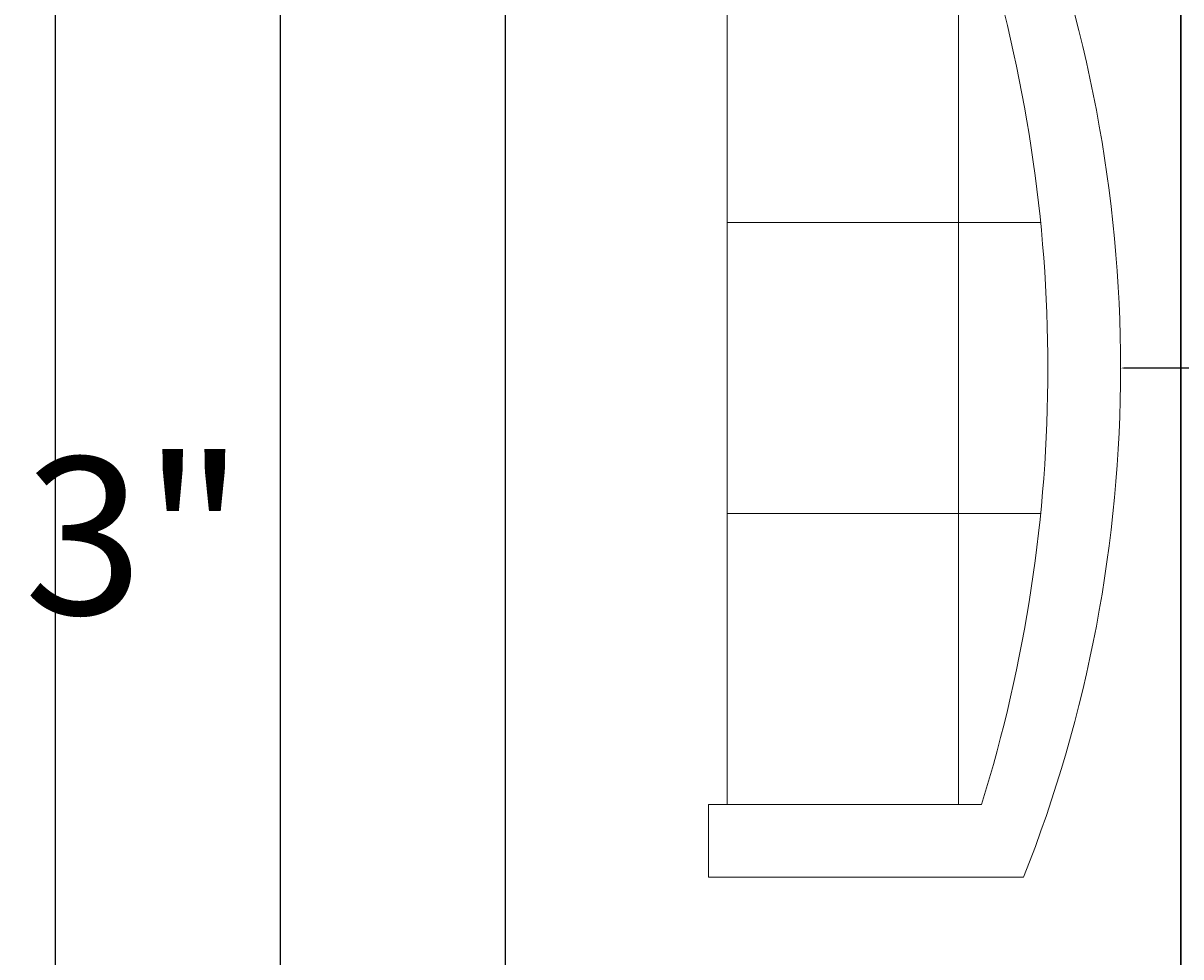
# Model space of a CAD drawing. Units: feet. Extents: x 1654 to 2985, y 1348 to 2230.
# Tile 47 of 53: x 2723 to 2785, y 1792 to 1842. Entities that reach past the tile are written whole.
import ezdxf

# ---------------------------------------------------------------- set-up
doc = ezdxf.new("R2010")
doc.units = ezdxf.units.FT
for name, color, linetype, lineweight in [('A-ANNO-DIMS', 2, 'Continuous', 18), ('A-AREA-IDEN', 7, 'Continuous', 18), ('A-FURN', 8, 'Continuous', 13)]:
    doc.layers.add(name, color=color, linetype=linetype, lineweight=lineweight)
doc.styles.get("Standard").update_dxf_attribs({"font": 'arial.ttf'})
doc.dimstyles.get("Standard").update_dxf_attribs({"dimtxt": 0.18, "dimasz": 0.18, "dimexe": 0.18, "dimexo": 0.0625, "dimgap": 0.09, "dimtad": 0, "dimtih": 1, "dimtoh": 1, "dimdec": 4, "dimzin": 0, "dimdsep": 46, "dimtxsty": 'Standard', "dimcen": 0.09, "dimadec": 0, "dimazin": 0, "dimtfac": 1, "dimtdec": 4, "dimtofl": 0, "dimtmove": 0, "dimatfit": 3, "dimfxl": 1, "dimtolj": 1, "dimtzin": 0, "dimarcsym": 0})

# ---------------------------------------------------------------- blocks, each defined once
blk = doc.blocks.new('Sofa - Roundback 7 ft.')
for p, q in [((-12.00002, -32.4421), (-12.00003, -6.5971)), ((11.99997, -32.4421), (11.99998, -6.5971)), ((-36.000027, -34), (-36.000027, -11.4696)), ((35.99998, -34), (35.99998, -11.4696)), ((-35.999844, -13.3819), (35.9998, -13.3819)), ((-36.000027, -32.4421), (35.99998, -32.4421))]:
    blk.add_line(p, q)
for points in [[(-36.000027, -34), (-42.000027, -34), (-42.000027, -8)], [(41.99998, -8), (41.99998, -34), (35.99998, -34)]]:
    blk.add_lwpolyline(points)
for centre, radius, start, end in [((0, -114.25), 114.25, 68.43141, 111.5686), ((-0.00001, -127.1968), 121.1968, 72.72033, 107.2797)]:
    blk.add_arc(centre, radius, start, end)
blk = doc.blocks.new('*D82')
at = {"layer": 'A-ANNO-DIMS', "color": 0, "lineweight": -2, "transparency": 16777216}
for p, q in [((2652.706, 2039.192), (2652.706, 1490.625)), ((2784.706, 2039.192), (2784.706, 1490.625)), ((2652.886, 1490.805), (2718.426, 1490.805)), ((2784.526, 1490.805), (2718.985, 1490.805))]:
    blk.add_line(p, q, dxfattribs=at)
at = {"layer": 'A-ANNO-DIMS', "color": 0, "transparency": 16777216}
for points in [[(2652.886, 1490.835), (2652.886, 1490.775), (2652.706, 1490.805)], [(2784.526, 1490.835), (2784.526, 1490.775), (2784.706, 1490.805)]]:
    blk.add_solid(points, dxfattribs=at)
at = {"layer": 'Defpoints', "color": 0, "transparency": 16777216}
for p in [(2652.706, 2039.255), (2784.706, 2039.255), (2784.706, 1490.805)]:
    blk.add_point(p, dxfattribs=at)
at = {"layer": 'A-ANNO-DIMS', "color": 0, "transparency": 16777216, "insert": (2718.706, 1490.805), "char_height": 0.18, "attachment_point": 5}
blk.add_mtext('\\A1;132', dxfattribs=at)
blk = doc.blocks.new('*D86')
at = {"layer": 'A-ANNO-DIMS', "color": 0, "lineweight": -2, "transparency": 16777216}
for p, q in [((2748.706, 1616.317), (2748.706, 2149.885)), ((2784.706, 1607.317), (2784.706, 2149.885)), ((2748.886, 2149.705), (2766.487, 2149.705)), ((2784.526, 2149.705), (2766.925, 2149.705))]:
    blk.add_line(p, q, dxfattribs=at)
at = {"layer": 'A-ANNO-DIMS', "color": 0, "transparency": 16777216}
for points in [[(2748.886, 2149.735), (2748.886, 2149.675), (2748.706, 2149.705)], [(2784.526, 2149.735), (2784.526, 2149.675), (2784.706, 2149.705)]]:
    blk.add_solid(points, dxfattribs=at)
at = {"layer": 'Defpoints', "color": 0, "transparency": 16777216}
for p in [(2784.706, 2149.705), (2748.706, 1616.255), (2784.706, 1607.255)]:
    blk.add_point(p, dxfattribs=at)
at = {"layer": 'A-ANNO-DIMS', "color": 0, "transparency": 16777216, "insert": (2766.706, 2149.705), "char_height": 0.18, "attachment_point": 5}
blk.add_mtext('\\A1;36', dxfattribs=at)
blk = doc.blocks.new('*D87')
at = {"layer": 'A-ANNO-DIMS', "color": 0, "lineweight": -2, "transparency": 16777216}
for p, q in [((2724.706, 1565.317), (2724.706, 2149.885)), ((2736.706, 1565.317), (2736.706, 2149.885)), ((2724.886, 2149.705), (2730.496, 2149.705)), ((2736.526, 2149.705), (2730.915, 2149.705))]:
    blk.add_line(p, q, dxfattribs=at)
at = {"layer": 'A-ANNO-DIMS', "color": 0, "transparency": 16777216}
for points in [[(2724.886, 2149.735), (2724.886, 2149.675), (2724.706, 2149.705)], [(2736.526, 2149.735), (2736.526, 2149.675), (2736.706, 2149.705)]]:
    blk.add_solid(points, dxfattribs=at)
at = {"layer": 'Defpoints', "color": 0, "transparency": 16777216}
for p in [(2736.706, 2149.705), (2724.706, 1565.255), (2736.706, 1565.255)]:
    blk.add_point(p, dxfattribs=at)
at = {"layer": 'A-ANNO-DIMS', "color": 0, "transparency": 16777216, "insert": (2730.706, 2149.705), "char_height": 0.18, "attachment_point": 5}
blk.add_mtext('\\A1;12', dxfattribs=at)
blk = doc.blocks.new('*D109')
at = {"layer": 'A-ANNO-DIMS', "color": 0, "lineweight": -2, "transparency": 16777216}
for p, q in [((2707.544, 1823.581), (2707.724, 1823.581)), ((2707.634, 1823.491), (2707.634, 1823.671)), ((2825.812, 1823.581), (2781.675, 1823.581))]:
    blk.add_line(p, q, dxfattribs=at)
at = {"layer": 'A-ANNO-DIMS', "color": 0, "transparency": 16777216}
blk.add_solid([(2781.675, 1823.611), (2781.675, 1823.551), (2781.495, 1823.581)], dxfattribs=at)
at = {"layer": 'Defpoints', "color": 0, "transparency": 16777216}
for p in [(2707.634, 1823.581), (2781.495, 1823.581)]:
    blk.add_point(p, dxfattribs=at)
at = {"layer": 'A-ANNO-DIMS', "color": 0, "transparency": 16777216, "insert": (2826.486, 1823.581), "char_height": 0.18, "attachment_point": 5}
blk.add_mtext('\\A1;2X R73.86', dxfattribs=at)

msp = doc.modelspace()

# ---------------------------------------------------------------- block references
at = {"layer": 'A-FURN', "xscale": 0.6464854603293951, "yscale": 0.6464854603293951, "zscale": 0.6464854603293951, "rotation": 270}
msp.add_blockref('Sofa - Roundback 7 ft.', (2781.495, 1823.581), dxfattribs=at)

# ---------------------------------------------------------------- texts
at = {"layer": 'A-AREA-IDEN'}
msp.add_text('11\'X11\'3"', height=8.38114, dxfattribs=at).set_placement((2684.7392, 1810.4431))

# ---------------------------------------------------------------- dimensions: what is measured, and where the dimension line sits
at = {"layer": 'A-ANNO-DIMS'}
for base, p1, p2, picture, middle in [((2736.7058, 2149.7049), (2724.7058, 1565.2549), (2736.7058, 1565.2549), '*D87', (2730.7058, 2149.7049)), ((2784.7058, 2149.7049), (2748.7058, 1616.2549), (2784.7058, 1607.2549), '*D86', (2766.7058, 2149.7049)), ((2784.7058, 1490.8049), (2652.7058, 2039.2549), (2784.7058, 2039.2549), '*D82', (2718.7058, 1490.8049))]:
    dim = msp.add_linear_dim(base=base, p1=p1, p2=p2, dimstyle='Standard', override={"dimdec": 0, "dimlfac": 1, "dimrnd": 0, "dimzin": 0, "dimdsep": 46, "dimlunit": 2}, dxfattribs=at)
    dim.commit()
    dim.dimension.update_dxf_attribs({"geometry": picture, "text_midpoint": middle})
dim = msp.add_radius_dim(center=(2707.634, 1823.581), mpoint=(2781.495, 1823.581), text='2X <>', dimstyle='Standard', override={"dimdec": 2, "dimlfac": 1, "dimrnd": 0, "dimzin": 0, "dimdsep": 46, "dimlunit": 2}, dxfattribs=at)
dim.commit()
dim.dimension.update_dxf_attribs({"geometry": '*D109', "text_midpoint": (2825.8115, 1823.581), "dimtype": 164})

doc.saveas('drawing.dxf')
